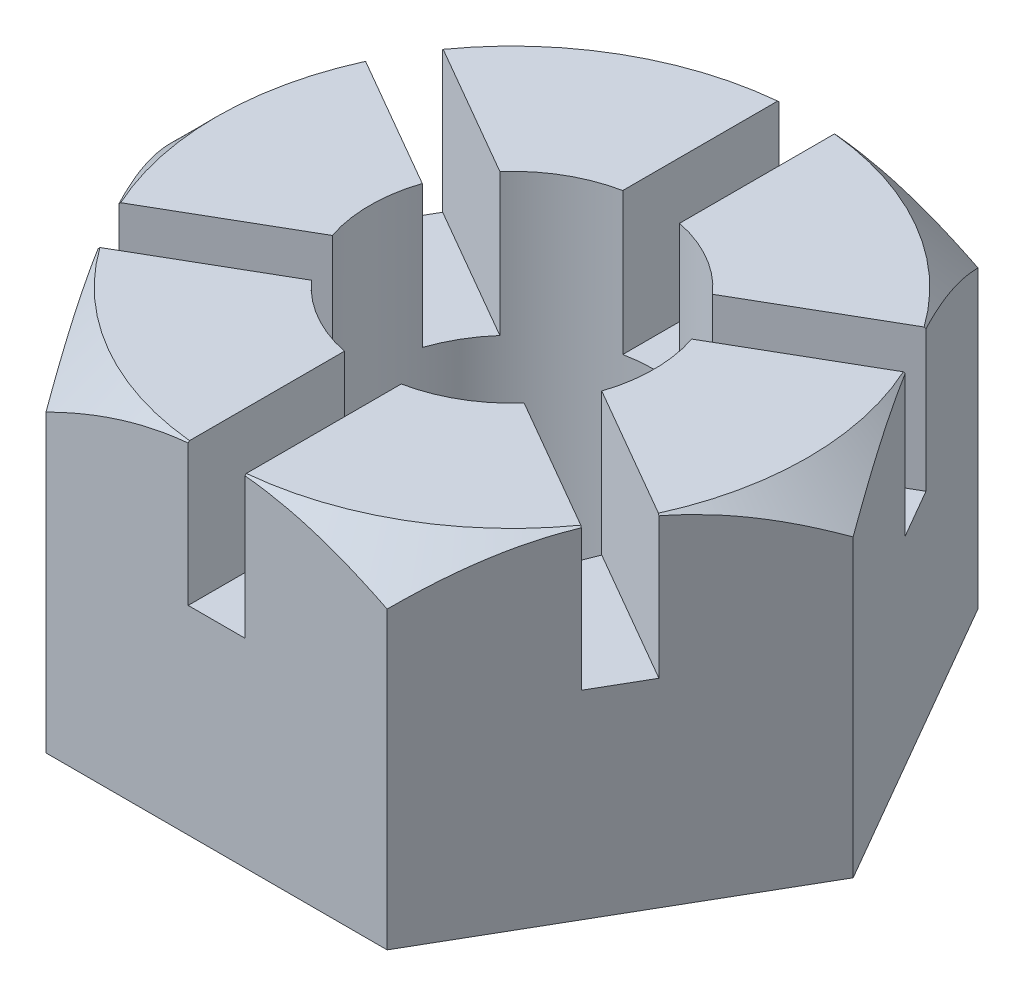
SolidWorks part; units mm, degrees
material "Plain Carbon Steel"
ref_plane "Front Plane" through (0, 0, 0) normal (0, 0, 1) x (1, 0, 0)
ref_plane "Top Plane" through (0, 0, 0) normal (0, 1, 0) x (1, 0, 0)
ref_plane "Right Plane" through (0, 0, 0) normal (1, 0, 0) x (0, 0, -1)
sketch "Hex Profile Sketch" plane through (0, 0, 0) normal (0, 1, 0) x (1, 0, 0)
  line L1 (30.0222, -52) -> (60.0444, 0)
  line L2 (60.0444, 0) -> (30.0222, 52)
  line L3 (30.0222, 52) -> (-30.0222, 52)
  line L4 (-30.0222, 52) -> (-60.0444, 0)
  line L5 (-60.0444, 0) -> (-30.0222, -52)
  line L6 (-30.0222, -52) -> (30.0222, -52)
  circle A0 centre (0, 0) radius 52 construction
  dimension "D1" = 104
extrude "Hex Body 104AF x 60" add sketch "Hex Profile Sketch" along normal blind 60
sketch "Crown Chamfer Sketch" plane through (0, 60, 0) normal (0, 1, 0) x (1, 0, 0)
  line L0 (-30.0222, -52) -> (30.0222, -52) construction
  circle A0 centre (0, 0) radius 52
extrude "Crown Chamfer 45deg" cut sketch "Crown Chamfer Sketch" against normal blind 60 draft 45 flip side to cut
sketch "Bore Sketch Ø50" plane through (0, 60, 0) normal (0, 1, 0) x (1, 0, 0)
  circle A0 centre (0, 0) radius 25
  dimension "D1" = 50
extrude "Bore Ø50" cut sketch "Bore Sketch Ø50" against normal blind 60
sketch "Castle Slots Sketch" plane through (0, 60, 0) normal (0, 1, 0) x (1, 0, 0)
  line L0 (-30.0222, -52) -> (0, -52) construction
  line L2 (-5, -24.4949) -> (-5, -52)
  line L4 (5, -24.4949) -> (5, -52)
  line L5 (0, -52) -> (30.0222, -52) construction
  line L6 (-5, -52) -> (0, -52)
  line L7 (0, -52) -> (5, -52)
  line L8 (-23.7132, -7.9173) -> (-47.5333, -21.6699)
  line L9 (-18.7132, -16.5776) -> (-42.5333, -30.3301)
  line L10 (-47.5333, -21.6699) -> (-45.0333, -26)
  line L11 (-45.0333, -26) -> (-42.5333, -30.3301)
  line L12 (-18.7132, 16.5776) -> (-42.5333, 30.3301)
  line L13 (-23.7132, 7.9173) -> (-47.5333, 21.6699)
  line L14 (-42.5333, 30.3301) -> (-45.0333, 26)
  line L15 (-45.0333, 26) -> (-47.5333, 21.6699)
  line L16 (5, 24.4949) -> (5, 52)
  line L17 (-5, 24.4949) -> (-5, 52)
  line L18 (5, 52) -> (0, 52)
  line L19 (0, 52) -> (-5, 52)
  line L20 (23.7132, 7.9173) -> (47.5333, 21.6699)
  line L21 (18.7132, 16.5776) -> (42.5333, 30.3301)
  line L22 (47.5333, 21.6699) -> (45.0333, 26)
  line L23 (45.0333, 26) -> (42.5333, 30.3301)
  line L24 (18.7132, -16.5776) -> (42.5333, -30.3301)
  line L25 (23.7132, -7.9173) -> (47.5333, -21.6699)
  line L26 (42.5333, -30.3301) -> (45.0333, -26)
  line L27 (45.0333, -26) -> (47.5333, -21.6699)
  circle A0 centre (0, 0) radius 25 construction
  arc A1 (-5, -24.4949) -> (5, -24.4949) centre (0, 0) ccw
  arc A2 (-23.7132, -7.9173) -> (-18.7132, -16.5776) centre (0, 0) ccw
  arc A3 (-18.7132, 16.5776) -> (-23.7132, 7.9173) centre (0, 0) ccw
  arc A4 (5, 24.4949) -> (-5, 24.4949) centre (0, 0) ccw
  arc A5 (23.7132, 7.9173) -> (18.7132, 16.5776) centre (0, 0) ccw
  arc A6 (18.7132, -16.5776) -> (23.7132, -7.9173) centre (0, 0) ccw
  point P37 (0, 0)
  dimension "D1" = 6
  dimension "D2" = 10
extrude "Castle Slots 6x10" cut sketch "Castle Slots Sketch" against normal blind 25
